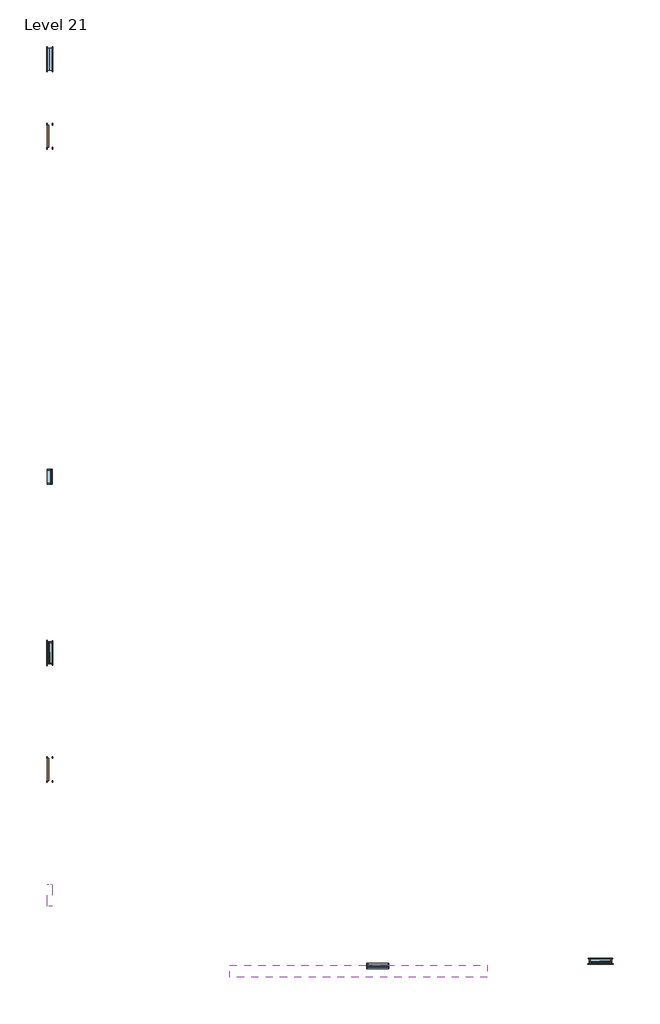
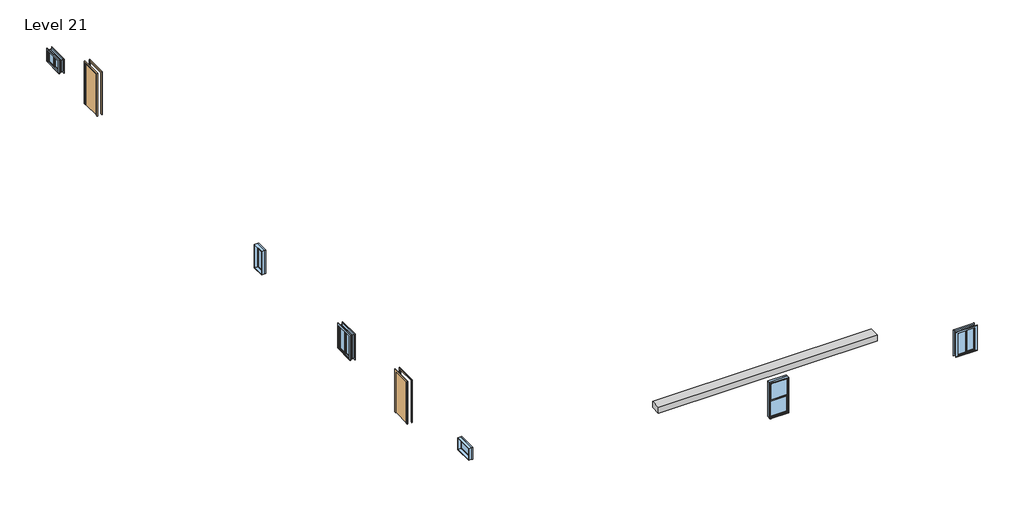
# One storey: 6 windows, 2 doors, 1 proxy.
"""IFC4 building model written with IfcOpenShell, lengths in millimetres."""

from ifc_helpers import new_model, si_unit, origin, place, context, project, spatial, transform, mapped, element, save
from components import generic_models_1_generic_models_1_77739e1a, door_54dd4da4, window_f274a882, window_80bd9af0, window_57c3ee1c, window_a4355bb3, window_54100e87

model = new_model("IFC4")

# Units and contexts
model_context = context("Model", 3, world=origin())
ifc_project = project(units=[si_unit("LENGTHUNIT", "METRE", prefix="MILLI")], contexts=[model_context])

# Site, building, storey
site = spatial("IfcSite", under=ifc_project)
building = spatial("IfcBuilding", under=site)
storey = spatial("IfcBuildingStorey", under=building, Name="Level 21", Elevation=33223.2)

# Proxy
placement = place(None, origin())
generic_models_1_generic_models_1_shape = generic_models_1_generic_models_1_77739e1a(model_context)
element("IfcBuildingElementProxy", 1, Name="Generic Models 1 : Generic Models 1", ObjectType="Generic Models 1 : Generic Models 1", at=placement, inside=storey, context=model_context, shape_type="MappedRepresentation", body=[
    mapped(generic_models_1_generic_models_1_shape, transform((0.0, 0.0, 0.0), x_axis=(1.0, 0.0, 0.0), y_axis=(0.0, 1.0, 0.0), z_axis=(0.0, 0.0, 1.0))),
])

# Doors
door_shape = door_54dd4da4(model_context)
element("IfcDoor", 2, ObjectType="Single-Flush : 36\" x 84\"", at=placement, inside=storey, context=model_context, shape_type="MappedRepresentation", body=[
    mapped(door_shape, transform((-15175.038074, 13495.0014639, 33223.2), x_axis=(0.0, 1.0, 0.0), y_axis=(-1.0, 0.0, 0.0), z_axis=(0.0, 0.0, 1.0))),
])
element("IfcDoor", 3, ObjectType="Single-Flush : 36\" x 84\"", at=placement, inside=storey, context=model_context, shape_type="MappedRepresentation", body=[
    mapped(door_shape, transform((-15175.038074, -12785.7915889, 33223.2), x_axis=(0.0, 1.0, 0.0), y_axis=(-1.0, 0.0, 0.0), z_axis=(0.0, 0.0, 1.0))),
])

# Windows
window_shape = window_f274a882(model_context)
element("IfcWindow", 4, ObjectType="Double Hung : 36\" x 72\"", at=placement, inside=storey, context=model_context, shape_type="MappedRepresentation", body=[
    mapped(window_shape, transform((-1560.638074, -20921.9985361, 33223.2), x_axis=(-1.0, 0.0, 0.0), y_axis=(0.0, -1.0, 0.0), z_axis=(0.0, 0.0, 1.0))),
])
window_2_shape = window_80bd9af0(model_context)
element("IfcWindow", 5, ObjectType="Fixed : 24\" x 48\"", at=placement, inside=storey, context=model_context, shape_type="MappedRepresentation", body=[
    mapped(window_2_shape, transform((-15175.038074, -670.9213044, 32510.818592), x_axis=(0.0, -1.0, 0.0), y_axis=(1.0, 0.0, 0.0), z_axis=(0.0, 0.0, 1.0))),
])
window_3_shape = window_57c3ee1c(model_context)
element("IfcWindow", 6, ObjectType="Fixed : 36\" x 24\"", at=placement, inside=storey, context=model_context, shape_type="MappedRepresentation", body=[
    mapped(window_3_shape, transform((-15175.038074, -18041.8099202, 33545.665757), x_axis=(0.0, -1.0, 0.0), y_axis=(1.0, 0.0, 0.0), z_axis=(0.0, 0.0, 1.0))),
])
window_4_shape = window_a4355bb3(model_context)
element("IfcWindow", 7, ObjectType="Slider with Trim : 36\" x 24\"", at=placement, inside=storey, context=model_context, shape_type="MappedRepresentation", body=[
    mapped(window_4_shape, transform((-15175.038074, 16695.4014639, 32568.765286), x_axis=(0.0, 1.0, 0.0), y_axis=(-1.0, 0.0, 0.0), z_axis=(0.0, 0.0, 1.0))),
])
window_5_shape = window_54100e87(model_context)
element("IfcWindow", 8, ObjectType="Slider with Trim : 36\" x 48\"", at=placement, inside=storey, context=model_context, shape_type="MappedRepresentation", body=[
    mapped(window_5_shape, transform((7684.961926, -20744.1985361, 32482.9595091), x_axis=(-1.0, 0.0, 0.0), y_axis=(0.0, -1.0, 0.0), z_axis=(0.0, 0.0, 1.0))),
])
element("IfcWindow", 9, ObjectType="Slider with Trim : 36\" x 48\"", at=placement, inside=storey, context=model_context, shape_type="MappedRepresentation", body=[
    mapped(window_5_shape, transform((-15175.038074, -7948.0213044, 32673.7666062), x_axis=(0.0, 1.0, 0.0), y_axis=(-1.0, 0.0, 0.0), z_axis=(0.0, 0.0, 1.0))),
])

save(model, "model.ifc")

# Revit data of these elements
# Type "Single-Flush : 36\" x 84\""
#   Type Mark = "1"
#   Construction Type Id = "MDOOR"
#   Assembly Code = "C1020"
#   Analytic Construction = "Metal"
#   Thickness = 0' - 2"
#   Heat Transfer Coefficient (U) = 0.651978 BTU/(h·ft²·°F)
#   Height = 7' - 0"
#   Trim Projection Ext = 0' - 1"
#   Trim Projection Int = 0' - 1"
#   Trim Width = 0' - 3"
#   Width = 3' - 0"
#   Define Thermal Properties by = 1
#   Door Material = Door - Panel
#   Frame Material = Door - Frame
#   Visual Light Transmittance = 0
#   Solar Heat Gain Coefficient = 0
#   Function = (empty or 0)
#   Wall Closure = (empty or 0)
# Type "Double Hung : 36\" x 72\""
#   Type Mark = "18"
#   Construction Type Id = "GSP4R"
#   Assembly Code = "B2020100"
#   Analytic Construction = "1/8 in Pilkington single glazing"
#   Visual Light Transmittance = 0.9
#   Solar Heat Gain Coefficient = 0.78
#   Heat Transfer Coefficient (U) = 0.6496 BTU/(h·ft²·°F)
#   Height = 6' - 0"
#   Default Sill Height = 1' - 0"
#   Width = 3' - 0"
#   Window Inset = 0' - 0 3/4"
#   Define Thermal Properties by = 1
#   Glass Pane Material = Glass
#   Sash Material = Sash
#   Description = (empty or 0)
#   Wall Closure = (empty or 0)
# Type "Fixed : 24\" x 48\""
#   Type Mark = "2"
#   Construction Type Id = "GSP4R"
#   Assembly Code = "B2020100"
#   Analytic Construction = "1/8 in Pilkington single glazing"
#   Visual Light Transmittance = 0.9
#   Solar Heat Gain Coefficient = 0.78
#   Heat Transfer Coefficient (U) = 0.6496 BTU/(h·ft²·°F)
#   Height = 4' - 0"
#   Default Sill Height = 3' - 0"
#   Width = 2' - 0"
#   Window Inset = 0' - 0 3/4"
#   Define Thermal Properties by = 1
#   Glass Pane Material = Glass
#   Sash Material = Sash
#   Wall Closure = (empty or 0)
# Type "Fixed : 36\" x 24\""
#   Type Mark = "8"
#   Construction Type Id = "GSP4R"
#   Assembly Code = "B2020100"
#   Analytic Construction = "1/8 in Pilkington single glazing"
#   Visual Light Transmittance = 0.9
#   Solar Heat Gain Coefficient = 0.78
#   Heat Transfer Coefficient (U) = 0.6496 BTU/(h·ft²·°F)
#   Height = 2' - 0"
#   Default Sill Height = 3' - 0"
#   Width = 3' - 0"
#   Window Inset = 0' - 0 3/4"
#   Define Thermal Properties by = 1
#   Glass Pane Material = Glass
#   Sash Material = Sash
#   Wall Closure = (empty or 0)
# Type "Slider with Trim : 36\" x 24\""
#   Type Mark = "23"
#   Construction Type Id = "GSP4R"
#   Assembly Code = "B2020100"
#   Analytic Construction = "1/8 in Pilkington single glazing"
#   Visual Light Transmittance = 0.9
#   Solar Heat Gain Coefficient = 0.78
#   Heat Transfer Coefficient (U) = 0.6496 BTU/(h·ft²·°F)
#   Height = 2' - 0"
#   Default Sill Height = 3' - 0"
#   Trim Projection - Ext. = 0' - 0 3/4"
#   Trim Projection - Int. = 0' - 0 3/4"
#   Trim Width - Exterior = 0' - 3 1/2"
#   Trim Width - Interior = 0' - 3 1/2"
#   Width = 3' - 0"
#   Window Inset = 0' - 0 3/4"
#   Define Thermal Properties by = 1
#   Glass Pane Material = Glass
#   Sash Material = Sash
#   Trim Exterior Material = Trim
#   Trim Interior Material = Trim
#   Wall Closure = (empty or 0)
# Type "Slider with Trim : 36\" x 48\""
#   Type Mark = "22"
#   Construction Type Id = "GSP4R"
#   Assembly Code = "B2020100"
#   Analytic Construction = "1/8 in Pilkington single glazing"
#   Visual Light Transmittance = 0.9
#   Solar Heat Gain Coefficient = 0.78
#   Heat Transfer Coefficient (U) = 0.6496 BTU/(h·ft²·°F)
#   Height = 4' - 0"
#   Default Sill Height = 3' - 0"
#   Trim Projection - Ext. = 0' - 0 3/4"
#   Trim Projection - Int. = 0' - 0 3/4"
#   Trim Width - Exterior = 0' - 3 1/2"
#   Trim Width - Interior = 0' - 3 1/2"
#   Width = 3' - 0"
#   Window Inset = 0' - 0 3/4"
#   Define Thermal Properties by = 1
#   Glass Pane Material = Glass
#   Sash Material = Sash
#   Trim Exterior Material = Trim
#   Trim Interior Material = Trim
#   Wall Closure = (empty or 0)
# Element 1 (IfcBuildingElementProxy, "Generic Models 1 : Generic Models 1")
#   Phase Created = New Construction
# Elements 2, 3 (IfcDoor, "Single-Flush : 36\" x 84\"")
#   Phase Created = New Construction
#   Materials on its faces: "Door - Frame", "Door - Panel"
# Element 4 (IfcWindow, "Double Hung : 36\" x 72\"")
#   Mark = "2"
#   Phase Created = New Construction
#   Materials on its faces: "Sash", "Glass"
# Element 5 (IfcWindow, "Fixed : 24\" x 48\"")
#   Mark = "46"
#   Phase Created = New Construction
#   Materials on its faces: "Sash", "Glass"
# Element 6 (IfcWindow, "Fixed : 36\" x 24\"")
#   Mark = "68"
#   Phase Created = New Construction
#   Materials on its faces: "Sash", "Glass"
# Element 7 (IfcWindow, "Slider with Trim : 36\" x 24\"")
#   Mark = "57"
#   Phase Created = New Construction
#   Materials on its faces: "Sash", "Trim", "Glass"
# Element 8 (IfcWindow, "Slider with Trim : 36\" x 48\"")
#   Mark = "24"
#   Phase Created = New Construction
#   Materials on its faces: "Sash", "Trim", "Glass"
# Element 9 (IfcWindow, "Slider with Trim : 36\" x 48\"")
#   Mark = "35"
#   Phase Created = New Construction
#   Materials on its faces: "Sash", "Trim", "Glass"
# Materials
#   "Door - Panel": class "Wood", colour RGB 210 159 95, transparency 0
#   "Door - Frame": colour RGB 118 70 51, transparency 0
#   "Glass": class "Glass", colour RGB 0 128 192, transparency 0.75, Description = "Soda Lime Glass", Cost = 0
#   "Sash": class "Wood", colour RGB 224 178 126, transparency 0
#   "Trim": class "Wood", colour RGB 224 178 126, transparency 0
